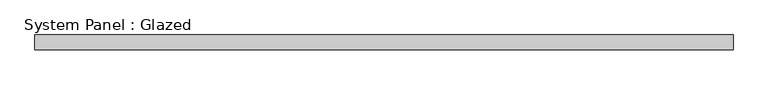
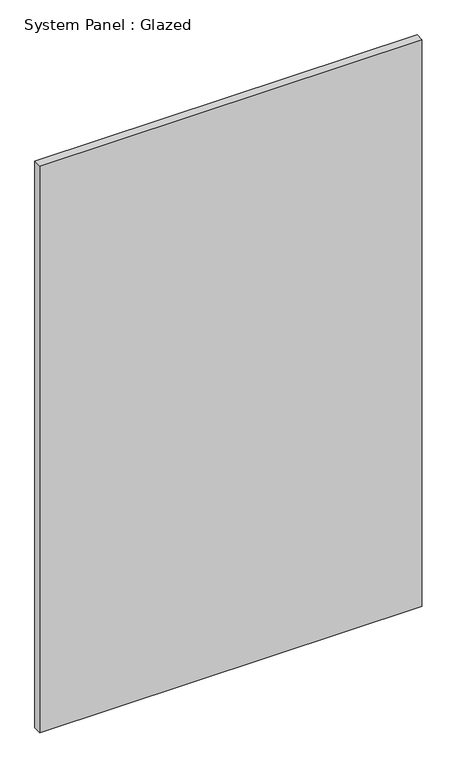
"""IFC4 building model written with IfcOpenShell, lengths in millimetres: plate geometry, System Panel : Glazed."""

from ifc_helpers import new_model, si_unit, origin, origin_with_axes, place, context, project, spatial, polyline, outline, extrude, source, transform, mapped, element, save


def system_panel_glazed_f54daf4a(model_context):
    return source(origin(), model_context, "Body", "SweptSolid", [
        extrude(outline(polyline([(600.075, 19.05), (-600.075, 19.05), (-600.075, 44.45), (600.075, 44.45), (600.075, 19.05)])), origin_with_axes(), (0.0, 0.0, 1.0), 1882.4971724),
    ])


if __name__ == "__main__":
    model = new_model("IFC4")
    model_context = context("Model", 3, world=origin())
    ifc_project = project(units=[si_unit("LENGTHUNIT", "METRE", prefix="MILLI")], contexts=[model_context])
    site = spatial("IfcSite", under=ifc_project)
    building = spatial("IfcBuilding", under=site)
    placement = place(None, origin())
    system_panel_glazed_shape = system_panel_glazed_f54daf4a(model_context)
    element("IfcPlate", 1, ObjectType="System Panel : Glazed", at=placement, inside=building, context=model_context, shape_type="MappedRepresentation", body=[
        mapped(system_panel_glazed_shape, transform((0.0, 0.0, 0.0), x_axis=(1.0, 0.0, 0.0), y_axis=(0.0, 1.0, 0.0), z_axis=(0.0, 0.0, 1.0))),
    ])
    save(model, "model.ifc")

# Revit data of these elements
# Type "System Panel : Glazed"
#   Construction Type Id = "GSP4R"
#   Analytic Construction = "1/8 in Pilkington single glazing"
#   Visual Light Transmittance = 0.9
#   Solar Heat Gain Coefficient = 0.86
#   Heat Transfer Coefficient (U) = 1.18115 BTU/(h·ft²·°F)
#   Define Thermal Properties by = 1
# Element 1 (IfcPlate, "System Panel : Glazed")
#   Materials on its faces: "Glass"
# Materials
#   "Glass": class "Glass", colour RGB 0 128 192, transparency 0.75, Description = "Soda Lime Glass", Cost = 0
